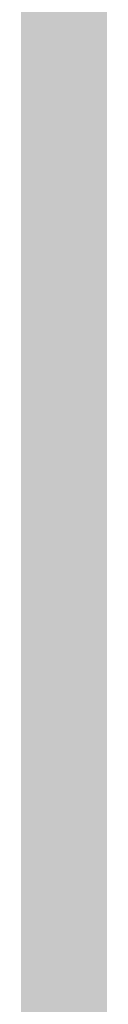
# Model space of a CAD drawing. Units: inches. Extents: x 2083 to 3317, y 1141 to 2115.
# Tile 189 of 256: x 3126.9283 to 3126.9467, y 1263.3548 to 1263.6134. Entities that reach past the tile are written whole.
import ezdxf

# ---------------------------------------------------------------- set-up
doc = ezdxf.new("R2010")
doc.units = ezdxf.units.IN
doc.layers.add('A-ANNO-DIMS', color=2, linetype='Continuous', lineweight=18)
doc.layers.add('A-WALL-PATT', color=251, linetype='Continuous', lineweight=13, true_color=0x636466)
doc.styles.get("Standard").update_dxf_attribs({"font": 'arial.ttf'})
doc.dimstyles.new('ISO-25', dxfattribs={"dimtxt": 12, "dimasz": 12, "dimexe": 1.25, "dimexo": 0.625, "dimtad": 1, "dimlunit": 3, "dimtxsty": 'Standard', "dimcen": 2.5, "dimadec": 0, "dimazin": 0, "dimtfac": 1, "dimtmove": 0, "dimatfit": 3, "dimfxl": 1, "dimarcsym": 0})

# ---------------------------------------------------------------- blocks, each defined once
blk = doc.blocks.new('*D26')
at = {"layer": 'A-ANNO-DIMS', "color": 0, "lineweight": -2, "transparency": 16777216}
for p, q in [((3088.98584, 1274.91509), (3088.98584, 1270.95196)), ((3111.24004, 1274.91509), (3111.24004, 1270.95196)), ((3076.98584, 1272.20196), (2840.26245, 1272.20196)), ((3111.24004, 1272.20196), (3088.98584, 1272.20196)), ((3123.24004, 1272.20196), (3135.24004, 1272.20196))]:
    blk.add_line(p, q, dxfattribs=at)
at = {"layer": 'A-ANNO-DIMS', "color": 0, "transparency": 16777216}
for points in [[(3076.98584, 1274.20196), (3076.98584, 1270.20196), (3088.98584, 1272.20196)], [(3123.24004, 1274.20196), (3123.24004, 1270.20196), (3111.24004, 1272.20196)]]:
    blk.add_solid(points, dxfattribs=at)
at = {"layer": 'Defpoints', "color": 0, "transparency": 16777216}
for p in [(3088.98584, 1275.54009), (3111.24004, 1275.54009), (3088.98584, 1272.20196)]:
    blk.add_point(p, dxfattribs=at)
at = {"layer": 'A-ANNO-DIMS', "color": 0, "transparency": 16777216, "insert": (2952.62415, 1279.0316), "char_height": 12, "attachment_point": 5}
blk.add_mtext('NIGHTSTAND 1\'-10 1/2" TYP.', dxfattribs=at)
blk = doc.blocks.new('*D27')
at = {"layer": 'A-ANNO-DIMS', "color": 0, "lineweight": -2, "transparency": 16777216}
for p, q in [((3114.57817, 1309.79428), (3114.57817, 1321.79428)), ((3111.86504, 1297.79428), (3115.82817, 1297.79428)), ((3114.57817, 1297.79428), (3114.57817, 1275.54009)), ((3111.86504, 1275.54009), (3115.82817, 1275.54009)), ((3114.57817, 1263.54009), (3114.57817, 1140.98859))]:
    blk.add_line(p, q, dxfattribs=at)
at = {"layer": 'A-ANNO-DIMS', "color": 0, "transparency": 16777216}
for points in [[(3112.57817, 1309.79428), (3116.57817, 1309.79428), (3114.57817, 1297.79428)], [(3112.57817, 1263.54009), (3116.57817, 1263.54009), (3114.57817, 1275.54009)]]:
    blk.add_solid(points, dxfattribs=at)
at = {"layer": 'Defpoints', "color": 0, "transparency": 16777216}
for p in [(3111.24004, 1297.79428), (3111.24004, 1275.54009), (3114.57817, 1275.54009)]:
    blk.add_point(p, dxfattribs=at)
at = {"layer": 'A-ANNO-DIMS', "color": 0, "transparency": 16777216, "insert": (3107.74853, 1196.26434), "char_height": 12, "attachment_point": 5, "rotation": 90}
blk.add_mtext('1\'-10 1/2" TYP.', dxfattribs=at)

msp = doc.modelspace()

# ---------------------------------------------------------------- hatches: boundary and pattern name
at = {"layer": 'A-WALL-PATT'}
h = msp.add_hatch(color=256, dxfattribs=at)
h.dxf.hatch_style = 1
h.paths.add_polyline_path([(3126.95978, 2020.76136), (2748.95978, 2020.76136), (2604.95978, 2020.76136), (2226.95978, 2020.76136), (2226.95978, 1702.76136), (2466.95978, 1702.76136), (2466.95978, 1582.76136), (2418.95978, 1582.76136), (2418.95978, 1477.76136), (2226.95978, 1477.76136), (2226.95978, 1263.26136), (2544.95978, 1263.26136), (2544.95978, 1411.76136), (2604.95978, 1411.76136), (2685.95978, 1411.76136), (2685.95978, 1420.76136), (2604.95978, 1420.76136), (2604.95978, 1573.76136), (2604.95978, 1702.76136), (2604.95978, 2011.76136), (2748.95978, 2011.76136), (2748.95978, 1702.76136), (2862.95978, 1702.76136), (2862.95978, 1621.76136), (2871.95978, 1621.76136), (2871.95978, 1702.76136), (2883.95978, 1702.76136), (2883.95978, 1706.93946, -0.026459), (2883.95978, 1711.76136), (2757.95978, 1711.76136), (2757.95978, 1807.76136), (2787.95978, 1807.76136), (2787.95978, 1812.26136), (2757.95978, 1812.26136), (2757.95978, 2011.76136), (2877.95978, 2011.76136), (2877.95978, 1812.26136), (2847.95978, 1812.26136), (2847.95978, 1807.76136), (2889.83574, 1807.76136), (2889.83574, 1812.26136), (2882.45978, 1812.26136), (2882.45978, 2011.76136), (3117.95978, 2011.76136), (3117.95978, 1812.26136), (2937.83574, 1812.26136), (2937.83574, 1807.76136), (2995.70978, 1807.76136), (2995.70978, 1796.11767), (3000.20978, 1796.11767), (3000.20978, 1807.76136), (3117.95978, 1807.76136), (3117.95978, 1711.76136), (3000.20978, 1711.76136), (3000.20978, 1760.11767), (2998.5727, 1760.11767, -0.020711), (2995.70978, 1760.11767), (2995.70978, 1711.76136), (2931.95978, 1711.76136), (2931.95978, 1702.76136), (3126.95978, 1702.76136)])
h.paths.add_polyline_path([(2471.45978, 2011.76136), (2471.45978, 1810.01136), (2462.71694, 1810.01136), (2462.71694, 1805.51136), (2505.95978, 1805.51136), (2505.95978, 1810.01136), (2475.95978, 1810.01136), (2475.95978, 2011.76136), (2595.95978, 2011.76136), (2595.95978, 1810.01136), (2565.95978, 1810.01136), (2565.95978, 1805.51136), (2595.95978, 1805.51136), (2595.95978, 1711.76136), (2235.95978, 1711.76136), (2235.95978, 1805.51136), (2353.70978, 1805.51136), (2353.70978, 1796.05416), (2358.20978, 1796.05416), (2358.20978, 1805.51136), (2414.71694, 1805.51136), (2414.71694, 1810.01136), (2235.95978, 1810.01136), (2235.95978, 2011.76136)], flags=16)
h.paths.add_polyline_path([(2270.20473, 1994.61001), (2270.20473, 1970.61001), (2246.20473, 1970.61001), (2246.20473, 1994.61001)], flags=0)
edge = h.paths.add_edge_path(flags=0)
edge.add_ellipse((2332.02739, 1899.79818), major_axis=(-3.04299, 3.04299), ratio=0.1682525, start_angle=-161.33217, end_angle=-156.30711, ccw=False)
edge.add_ellipse((2333.08204, 1898.74353), major_axis=(-1.05465, 1.05465), ratio=0.4535321, start_angle=-123.37102, end_angle=-94.15911)
edge = h.paths.add_edge_path(flags=0)
edge.add_ellipse((2332.02739, 1968.87629), major_axis=(3.04299, 3.04299), ratio=0.1682525, start_angle=18.66783, end_angle=23.69289)
edge.add_spline(control_points=[(2332.9256, 1970.6911), (2332.22677, 1970.3361), (2330.89371, 1969.65891), (2328.41308, 1970.93214), (2327.20393, 1967.74871), (2324.7096, 1969.95559), (2322.53282, 1967.01235), (2320.01285, 1971.29581), (2317.68031, 1968.15784), (2316.04053, 1967.10205), (2315.4269, 1966.8096)], knot_values=[0, 0, 0, 0, 2.267059, 4.324559, 6.685584, 8.878641, 11.121502, 14.300359, 17.755284, 19.732645, 19.732645, 19.732645, 19.732645], degree=3, periodic=0)
edge.add_ellipse((2332.02739, 1968.87629), major_axis=(3.04299, 3.04299), ratio=0.1682525, start_angle=18.66783, end_angle=23.69289, ccw=False)
edge.add_ellipse((2333.08204, 1969.93094), major_axis=(1.05465, 1.05465), ratio=0.4535321, start_angle=56.62898, end_angle=85.84089, ccw=False)
edge = h.paths.add_edge_path(flags=0)
edge.add_spline(control_points=[(2296.42829, 1967.98791), (2293.6278, 1965.33631), (2287.70362, 1959.72709), (2299.74386, 1949.9957), (2294.53259, 1935.66853), (2290.57323, 1920.60351), (2293.39412, 1909.97369), (2296.18541, 1904.96654)], knot_values=[0.099185, 0.099185, 0.099185, 0.099185, 0.345301, 0.619822, 0.982653, 1.386093, 1.810555, 1.810555, 1.810555, 1.810555], degree=3, periodic=0)
edge.add_spline(control_points=[(2296.18541, 1904.96654), (2297.38358, 1902.6193), (2298.00097, 1901.94931), (2298.55297, 1901.46815)], knot_values=[0.006246, 0.006246, 0.006246, 0.006246, 0.055476, 0.055476, 0.055476, 0.055476], degree=3, periodic=0)
edge.add_spline(control_points=[(2298.55297, 1901.46815), (2297.25861, 1900.92322), (2295.22529, 1900.23213), (2293.06023, 1900.61421), (2292.10142, 1900.78841), (2292.08958, 1900.79057)], knot_values=[0.312835, 0.312835, 0.312835, 0.312835, 0.40178, 0.474987, 0.475903, 0.475903, 0.475903, 0.475903], degree=3, periodic=0)
edge.add_arc((2292.79365, 1904.66411), 3.93701, 215.4209, 259.69818, ccw=False)
edge.add_spline(control_points=[(2289.58531, 1902.3823), (2289.47665, 1902.53509), (2289.36848, 1902.68804), (2289.26086, 1902.84117)], knot_values=[0.102872, 0.102872, 0.102872, 0.102872, 0.116896, 0.116896, 0.116896, 0.116896], degree=3, periodic=0)
edge.add_spline(control_points=[(2289.26086, 1902.84117), (2288.6866, 1902.55019), (2287.64005, 1902.0199), (2285.88134, 1901.87395), (2283.85297, 1901.50435), (2281.71999, 1899.71054), (2278.46699, 1899.49294), (2276.15714, 1901.8832), (2272.25895, 1899.80407), (2267.77761, 1901.84318), (2262.24388, 1900.18403), (2257.41493, 1901.78206), (2254.31837, 1900.72612), (2253.17828, 1900.33734)], knot_values=[0, 0, 0, 0, 1.907977, 3.477176, 5.261074, 7.972851, 11.680248, 13.717921, 16.939592, 22.789562, 27.502503, 33.595215, 37.145618, 37.145618, 37.145618, 37.145618], degree=3, periodic=0)
edge.add_line((2253.17828, 1900.33734), (2250.24424, 1902.84117))
edge.add_line((2250.24424, 1902.84117), (2250.24424, 1965.8333))
edge.add_line((2250.24424, 1965.8333), (2253.17828, 1968.33712))
edge.add_spline(control_points=[(2253.17828, 1968.33712), (2254.31837, 1967.94835), (2257.41493, 1966.89241), (2262.24388, 1968.49043), (2267.77761, 1966.83128), (2271.52673, 1968.53722), (2273.87591, 1967.82829), (2274.2067, 1967.72764)], knot_values=[0, 0, 0, 0, 0.09018, 0.244935, 0.364644, 0.513233, 0.537855, 0.537855, 0.537855, 0.537855], degree=3, periodic=0)
edge.add_arc((2274.35289, 1963.79335), 3.93701, 72.05113, 92.12795, ccw=False)
edge.add_arc((2281.29693, 1985.23), 18.5963, 252.051134, 288.565722)
edge.add_arc((2292.31672, 1956.02888), 12.64608, 71.026788, 113.778218, ccw=False)
edge = h.paths.add_edge_path(flags=0)
edge.add_spline(control_points=[(2274.89941, 1951.85619), (2275.06616, 1951.61659), (2275.23269, 1951.37659), (2275.39799, 1951.13585)], knot_values=[1.409916, 1.409916, 1.409916, 1.409916, 1.43159, 1.43159, 1.43159, 1.43159], degree=3, periodic=0)
edge.add_spline(control_points=[(2275.39799, 1951.13585), (2275.79211, 1950.56189), (2276.17923, 1949.98377), (2276.54555, 1949.3971)], knot_values=[1.358238, 1.358238, 1.358238, 1.358238, 1.409916, 1.409916, 1.409916, 1.409916], degree=3, periodic=0)
edge.add_line((2276.54555, 1949.3971), (2277.43729, 1947.86218))
edge.add_spline(control_points=[(2277.43729, 1947.86218), (2276.30383, 1945.67311), (2274.6397, 1942.42688), (2274.63161, 1938.0939), (2272.79912, 1930.85155), (2274.35643, 1943.89705), (2275.94768, 1947.92336), (2276.54555, 1949.3971)], knot_values=[0.005632, 0.005632, 0.005632, 0.005632, 0.186014, 0.266002, 0.357087, 0.59639, 0.739732, 0.739732, 0.739732, 0.739732], degree=3, periodic=0)
edge.add_spline(control_points=[(2276.54555, 1949.3971), (2276.17923, 1949.98377), (2275.79211, 1950.56189), (2275.39799, 1951.13585)], knot_values=[1.358238, 1.358238, 1.358238, 1.358238, 1.409916, 1.409916, 1.409916, 1.409916], degree=3, periodic=0)
edge.add_spline(control_points=[(2275.39799, 1951.13585), (2274.9425, 1950.08045), (2274.20776, 1948.02527), (2273.9346, 1944.85148), (2272.46853, 1937.62749), (2273.46622, 1945.69647), (2274.70062, 1951.05947), (2274.89941, 1951.85619)], knot_values=[0.104364, 0.104364, 0.104364, 0.104364, 0.189636, 0.269624, 0.36071, 0.600013, 0.644622, 0.644622, 0.644622, 0.644622], degree=3, periodic=0)
h.paths.add_polyline_path([(2269.16751, 1963.12757, -0.357527), (2268.17063, 1960.97637, -0.092561), (2268.17063, 1939.43632, -0.357527), (2269.16751, 1937.28512, -0.357527), (2267.01631, 1938.282, -0.164785), (2254.68558, 1938.282, -0.357527), (2252.53438, 1937.28512, -0.357527), (2253.53126, 1939.43632, -0.092561), (2253.53126, 1960.97637, -0.357527), (2252.53438, 1963.12757, -0.357527), (2254.68558, 1962.13069, -0.164785), (2267.01631, 1962.13069, -0.357527)], flags=0)
h.paths.add_polyline_path([(2248.87407, 1967.8018), (2248.87407, 1957.02771), (2249.45778, 1957.02771), (2249.45778, 1911.64676), (2248.87407, 1911.64676), (2248.87407, 1900.87267), (2246.51186, 1900.87267, 0.197327), (2244.14966, 1902.45687), (2244.14966, 1966.21759, 0.197327), (2246.51186, 1967.8018)], flags=0)
h.paths.add_polyline_path([(2269.16751, 1931.38934, -0.357527), (2268.17063, 1929.23814, -0.092561), (2268.17063, 1907.6981, -0.357527), (2269.16751, 1905.54689, -0.357527), (2267.01631, 1906.54377, -0.164785), (2254.68558, 1906.54377, -0.357527), (2252.53438, 1905.54689, -0.357527), (2253.53126, 1907.6981, -0.092561), (2253.53126, 1929.23814, -0.357527), (2252.53438, 1931.38934, -0.357527), (2254.68558, 1930.39246, -0.164785), (2267.01631, 1930.39246, -0.357527)], flags=0)
edge = h.paths.add_edge_path(flags=0)
edge.add_spline(control_points=[(2276.19686, 1906.7237), (2276.16814, 1909.02893), (2276.11405, 1913.37185), (2270.59842, 1924.92498), (2273.90517, 1919.01278), (2275.92171, 1916.26206), (2275.47457, 1912.40215), (2277.25787, 1910.38062), (2276.69604, 1908.22504), (2276.64622, 1906.81302), (2276.61782, 1906.00841)], knot_values=[0, 0, 0, 0, 8.61026, 16.221274, 18.843057, 23.804898, 27.440828, 29.356102, 31.203478, 33.650687, 33.650687, 33.650687, 33.650687], degree=3, periodic=0)
edge.add_spline(control_points=[(2276.61782, 1906.00841), (2276.62331, 1905.62414), (2276.49774, 1904.62866), (2275.44178, 1903.85473), (2274.93731, 1903.08045), (2274.85908, 1902.84117)], knot_values=[0.156488, 0.156488, 0.156488, 0.156488, 0.184398, 0.231376, 0.250598, 0.250598, 0.250598, 0.250598], degree=3, periodic=0)
edge.add_line((2274.85908, 1902.84117), (2276.50598, 1902.84117))
edge.add_spline(control_points=[(2276.50598, 1902.84117), (2276.78831, 1903.08494), (2277.66507, 1904.1252), (2278.24954, 1904.34074), (2277.65387, 1908.52739), (2278.15567, 1906.22781), (2278.10046, 1905.28595), (2278.84667, 1904.06901), (2277.85679, 1903.41495), (2277.87419, 1902.99105), (2277.90356, 1902.84117)], knot_values=[0.059574, 0.059574, 0.059574, 0.059574, 0.080753, 0.103741, 0.16972, 0.176036, 0.207137, 0.240474, 0.262341, 0.27366, 0.27366, 0.27366, 0.27366], degree=3, periodic=0)
edge.add_line((2277.90356, 1902.84117), (2280.02983, 1902.84117))
edge.add_spline(control_points=[(2280.02983, 1902.84117), (2279.88822, 1903.0884), (2279.49926, 1903.98155), (2280.15228, 1905.93935), (2278.10362, 1909.65776), (2279.76239, 1907.18529), (2280.3279, 1904.87486), (2280.48511, 1903.48959), (2281.46327, 1903.24943), (2281.75834, 1902.9365), (2281.83404, 1902.84117)], knot_values=[0.013856, 0.013856, 0.013856, 0.013856, 0.034874, 0.088867, 0.107879, 0.126738, 0.158714, 0.193757, 0.217487, 0.226722, 0.226722, 0.226722, 0.226722], degree=3, periodic=0)
edge.add_spline(control_points=[(2281.83404, 1902.84117), (2281.78753, 1902.8267), (2281.64702, 1902.78299), (2281.39553, 1902.85949), (2281.08808, 1902.98524), (2280.72068, 1903.0609), (2280.33345, 1903.02573), (2280.12477, 1902.89888), (2280.02983, 1902.84117)], knot_values=[0, 0, 0, 0, 0.14413, 0.435517, 0.749276, 1.153046, 1.548371, 1.878348, 1.878348, 1.878348, 1.878348], degree=3, periodic=0)
edge.add_line((2280.02983, 1902.84117), (2277.90356, 1902.84117))
edge.add_spline(control_points=[(2277.90356, 1902.84117), (2277.89286, 1902.79586), (2277.8654, 1902.67964), (2277.60748, 1902.68748), (2277.27405, 1902.8007), (2276.83792, 1902.61977), (2276.58381, 1902.78926), (2276.50598, 1902.84117)], knot_values=[0, 0, 0, 0, 0.127189, 0.326199, 0.628009, 1.24357, 1.515331, 1.515331, 1.515331, 1.515331], degree=3, periodic=0)
edge.add_line((2276.50598, 1902.84117), (2274.85908, 1902.84117))
edge.add_spline(control_points=[(2274.85908, 1902.84117), (2274.81444, 1902.89859), (2274.72513, 1903.01345), (2274.49348, 1903.11897), (2274.24429, 1902.96054), (2273.93712, 1903.18494), (2273.61404, 1902.98314), (2273.40832, 1902.88304), (2273.32225, 1902.84117)], knot_values=[0, 0, 0, 0, 0.21843, 0.436957, 0.687977, 0.990379, 1.398396, 1.69185, 1.69185, 1.69185, 1.69185], degree=3, periodic=0)
edge.add_spline(control_points=[(2273.32225, 1902.84117), (2273.61674, 1903.44569), (2274.274, 1904.53825), (2276.02724, 1904.5737), (2276.20696, 1906.58364), (2276.19686, 1906.7237)], knot_values=[0.012227, 0.012227, 0.012227, 0.012227, 0.059472, 0.106218, 0.134458, 0.134458, 0.134458, 0.134458], degree=3, periodic=0)
h.paths.add_polyline_path([(2270.77605, 1897.78983), (2270.77605, 1873.78983), (2246.77605, 1873.78983), (2246.77605, 1897.78983)], flags=0)
h.paths.add_polyline_path([(2353.70978, 1760.00506), (2353.70978, 1760.05416), (2358.20978, 1760.05416, -0.033729)], flags=0)
h.paths.add_polyline_path([(2321.81912, 1737.52919), (2341.99533, 1737.52919, -0.414214), (2343.20327, 1736.32124), (2343.20327, 1721.0206, -0.414214), (2341.99533, 1719.81265), (2321.81912, 1719.81265, -0.414214), (2320.61117, 1721.0206), (2320.61117, 1736.32124, -0.414214)], flags=0)
h.paths.add_polyline_path([(2324.23501, 1736.32124), (2339.57944, 1736.32124, -0.414214), (2341.99533, 1733.90535), (2341.99533, 1725.44973, -0.414214), (2339.57944, 1723.03384), (2333.68059, 1723.03384), (2333.84532, 1722.04547, -0.870646), (2335.4254, 1721.82589, -0.767327), (2333.92269, 1721.42324), (2331.29102, 1721.42324, -0.767327), (2329.78832, 1721.82589, -0.870646), (2331.3684, 1722.04547), (2331.53313, 1723.03384), (2324.23501, 1723.03384, -0.414214), (2321.81912, 1725.44973), (2321.81912, 1733.90535, -0.414214)], flags=0)
h.paths.add_polyline_path([(2570.48379, 1928.61544), (2589.68379, 1928.61544), (2590.16883, 1928.61544), (2590.16883, 1904.9934), (2570.48379, 1904.9934)], flags=0)
h.paths.add_polyline_path([(2574.44732, 1927.26382, -1), (2572.82884, 1927.26382, -1)], flags=0)
h.paths.add_polyline_path([(2573.08987, 1926.94088), (2573.92503, 1927.77604), (2574.14774, 1927.55333), (2573.31258, 1926.71817)], flags=0)
h.paths.add_polyline_path([(2578.77906, 1919.72962, -1), (2571.59166, 1919.72962, -1)], flags=0)
h.paths.add_polyline_path([(2578.38536, 1919.72962, -1), (2571.98536, 1919.72962, -1)], flags=0)
h.paths.add_polyline_path([(2331.59576, 1729.47622, -1), (2333.61795, 1729.47622, -1)], flags=0)
h.paths.add_polyline_path([(2578.03423, 1927.26382, -1), (2576.41574, 1927.26382, -1)], flags=0)
h.paths.add_polyline_path([(2576.68885, 1927.53109), (2576.91156, 1927.7538), (2577.74673, 1926.91863), (2577.52402, 1926.69592)], flags=0)
h.paths.add_polyline_path([(2578.13906, 1909.85954, -1), (2572.23166, 1909.85954, -1)], flags=0)
h.paths.add_polyline_path([(2577.74536, 1909.85954, -1), (2572.62536, 1909.85954, -1)], flags=0)
h.paths.add_polyline_path([(2583.79772, 1927.26382, -1), (2582.17923, 1927.26382, -1)], flags=0)
h.paths.add_polyline_path([(2582.71865, 1927.7538), (2583.55381, 1926.91863), (2583.3311, 1926.69592), (2582.49594, 1927.53109)], flags=0)
h.paths.add_polyline_path([(2582.49594, 1927.53109), (2582.71865, 1927.7538), (2583.55381, 1926.91863), (2583.3311, 1926.69592)], flags=0)
h.paths.add_polyline_path([(2587.73906, 1920.52962, -1), (2581.83166, 1920.52962, -1)], flags=0)
h.paths.add_polyline_path([(2587.34536, 1920.52962, -1), (2582.22536, 1920.52962, -1)], flags=0)
h.paths.add_polyline_path([(2587.38462, 1927.26382, -1), (2585.76613, 1927.26382, -1)], flags=0)
h.paths.add_polyline_path([(2586.08199, 1926.98025), (2586.91716, 1927.81541), (2587.13987, 1927.5927), (2586.3047, 1926.75754)], flags=0)
h.paths.add_polyline_path([(2588.37906, 1910.65954, -1), (2581.19166, 1910.65954, -1)], flags=0)
h.paths.add_polyline_path([(2587.98536, 1910.65954, -1), (2581.58536, 1910.65954, -1)], flags=0)
h.paths.add_polyline_path([(2417.16773, 1729.4779), (2437.34394, 1729.4779, -0.414214), (2438.55188, 1728.26995), (2438.55188, 1712.96931, -0.414214), (2437.34394, 1711.76136), (2417.16773, 1711.76136, -0.414214), (2415.95978, 1712.96931), (2415.95978, 1728.26995, -0.414214)], flags=0)
h.paths.add_polyline_path([(2419.58362, 1728.26995), (2434.92805, 1728.26995, -0.414214), (2437.34394, 1725.85406), (2437.34394, 1717.39844, -0.414214), (2434.92805, 1714.98255), (2429.0292, 1714.98255), (2429.19393, 1713.99418, -0.870646), (2430.77401, 1713.7746, -0.767327), (2429.2713, 1713.37195), (2426.63963, 1713.37195, -0.767327), (2425.13693, 1713.7746, -0.870646), (2426.71701, 1713.99418), (2426.88174, 1714.98255), (2419.58362, 1714.98255, -0.414214), (2417.16773, 1717.39844), (2417.16773, 1725.85406, -0.414214)], flags=0)
h.paths.add_polyline_path([(2419.58362, 1728.26995), (2434.92805, 1728.26995, -0.414214), (2437.34394, 1725.85406), (2437.34394, 1717.39844, -0.414214), (2434.92805, 1714.98255), (2429.0292, 1714.98255), (2428.35812, 1719.00903), (2427.55282, 1719.00903), (2426.88174, 1714.98255), (2419.58362, 1714.98255, -0.414214), (2417.16773, 1717.39844), (2417.16773, 1725.85406, -0.414214)], flags=0)
h.paths.add_polyline_path([(2426.94437, 1721.42492, -1), (2428.96656, 1721.42492, -1)], flags=0)
h.paths.add_polyline_path([(2475.95978, 1702.76136), (2595.95978, 1702.76136), (2595.95978, 1582.76136), (2475.95978, 1582.76136)], flags=16)
h.paths.add_polyline_path([(2427.95978, 1573.76136), (2595.95978, 1573.76136), (2595.95978, 1468.76136), (2595.95978, 1420.76136), (2384.45978, 1420.76136), (2384.45978, 1468.76136), (2427.95978, 1468.76136)], flags=16)
h.paths.add_polyline_path([(2379.95978, 1468.76136), (2379.95978, 1420.76136), (2235.95978, 1420.76136), (2235.95978, 1468.76136)], flags=16)
h.paths.add_polyline_path([(2317.816, 1466.69577), (2337.9922, 1466.69577, -0.414214), (2339.20015, 1465.48782), (2339.20015, 1450.18718, -0.414214), (2337.9922, 1448.97923), (2317.816, 1448.97923, -0.414214), (2316.60805, 1450.18718), (2316.60805, 1465.48782, -0.414214)], flags=0)
h.paths.add_polyline_path([(2320.23189, 1465.48782), (2335.57631, 1465.48782, -0.414214), (2337.9922, 1463.07193), (2337.9922, 1454.61631, -0.414214), (2335.57631, 1452.20042), (2329.67747, 1452.20042), (2329.84219, 1451.21205, -0.870646), (2331.42228, 1450.99247, -0.767327), (2329.91957, 1450.58983), (2327.2879, 1450.58983, -0.767327), (2325.7852, 1450.99247, -0.870646), (2327.36528, 1451.21205), (2327.53001, 1452.20042), (2320.23189, 1452.20042, -0.414214), (2317.816, 1454.61631), (2317.816, 1463.07193, -0.414214)], flags=0)
h.paths.add_polyline_path([(2320.23189, 1465.48782), (2335.57631, 1465.48782, -0.414214), (2337.9922, 1463.07193), (2337.9922, 1454.61631, -0.414214), (2335.57631, 1452.20042), (2329.67747, 1452.20042), (2329.00638, 1456.22691), (2328.20109, 1456.22691), (2327.53001, 1452.20042), (2320.23189, 1452.20042, -0.414214), (2317.816, 1454.61631), (2317.816, 1463.07193, -0.414214)], flags=0)
h.paths.add_polyline_path([(2327.59264, 1458.6428, -1), (2329.61483, 1458.6428, -1)], flags=0)
h.paths.add_polyline_path([(2244.41174, 1433.34045), (2241.92094, 1433.34045, -0.414214), (2240.01786, 1435.24354), (2240.01786, 1440.95281, -0.414211), (2241.92093, 1442.8559), (2244.41174, 1442.8559, -1.976472)], flags=0)
h.paths.add_polyline_path([(2245.35689, 1434.39754, -0.414214), (2245.35689, 1441.79881, -2.144098)], flags=0)
h.paths.add_polyline_path([(2535.95978, 1416.26136), (2535.95978, 1272.26136), (2235.95978, 1272.26136), (2235.95978, 1416.26136)], flags=16)
h.paths.add_polyline_path([(2260.11956, 1384.29284), (2260.11956, 1362.03865), (2237.86537, 1362.03865), (2237.86537, 1384.29284)], flags=0)
edge = h.paths.add_edge_path(flags=0)
edge.add_line((2318.25185, 1362.0933), (2318.1458, 1362.00097))
edge.add_ellipse((2317.44512, 1360.43104), major_axis=(2.82164, 2.82164), ratio=0.1682525, start_angle=18.66783, end_angle=20.94813, ccw=False)
edge.add_ellipse((2318.42305, 1361.40897), major_axis=(0.97793, 0.97793), ratio=0.4535321, start_angle=56.62898, end_angle=70.2262, ccw=False)
edge = h.paths.add_edge_path(flags=0)
edge.add_line((2319.10737, 1295.57108), (2319.01504, 1295.67713))
edge.add_ellipse((2317.44512, 1296.37781), major_axis=(-2.82164, 2.82164), ratio=0.1682525, start_angle=-161.33217, end_angle=-159.05187, ccw=False)
edge.add_ellipse((2318.42305, 1295.39988), major_axis=(-0.97793, 0.97793), ratio=0.4535321, start_angle=-123.37102, end_angle=-109.7738)
edge = h.paths.add_edge_path(flags=0)
edge.add_spline(control_points=[(2284.21035, 1301.17022), (2284.58069, 1300.44472), (2284.89119, 1299.89202), (2285.15955, 1299.46102)], knot_values=[0.039066, 0.039066, 0.039066, 0.039066, 0.055476, 0.055476, 0.055476, 0.055476], degree=3, periodic=0)
edge.add_line((2285.15955, 1299.46102), (2284.21035, 1301.17022))
edge = h.paths.add_edge_path(flags=0)
edge.add_line((2280.41246, 1297.29801), (2283.36999, 1297.03612))
edge.add_line((2283.36999, 1297.03612), (2286.40569, 1297.92631))
edge.add_spline(control_points=[(2286.40569, 1297.92631), (2285.30549, 1297.46312), (2284.34478, 1297.12915), (2283.36999, 1297.03612)], knot_values=[0.394369, 0.394369, 0.394369, 0.394369, 0.475903, 0.475903, 0.475903, 0.475903], degree=3, periodic=0)
edge.add_spline(control_points=[(2283.36999, 1297.03612), (2283.28139, 1297.02767), (2282.31629, 1296.95734), (2281.3125, 1297.13448), (2280.42344, 1297.29602), (2280.41246, 1297.29801)], knot_values=[0.312835, 0.312835, 0.312835, 0.312835, 0.320246, 0.393453, 0.394369, 0.394369, 0.394369, 0.394369], degree=3, periodic=0)
edge = h.paths.add_edge_path(flags=0)
edge.add_line((2284.43556, 1359.60729), (2280.44629, 1355.32805))
edge.add_line((2280.44629, 1355.32805), (2279.57999, 1351.01775))
edge.add_line((2279.57999, 1351.01775), (2282.41297, 1346.58043))
edge.add_spline(control_points=[(2282.41297, 1346.58043), (2283.15333, 1345.58924), (2284.2529, 1344.0289), (2284.80104, 1342.38717), (2284.93516, 1341.80554)], knot_values=[1.240098, 1.240098, 1.240098, 1.240098, 1.332892, 1.382712, 1.382712, 1.382712, 1.382712], degree=3, periodic=0)
edge.add_spline(control_points=[(2284.93516, 1341.80554), (2285.31911, 1340.1406), (2285.23303, 1338.4092), (2284.90994, 1336.65412)], knot_values=[1.097484, 1.097484, 1.097484, 1.097484, 1.240098, 1.240098, 1.240098, 1.240098], degree=3, periodic=0)
edge.add_spline(control_points=[(2284.90994, 1336.65412), (2284.58685, 1334.89904), (2284.02675, 1333.12027), (2283.46264, 1331.36058)], knot_values=[0.95487, 0.95487, 0.95487, 0.95487, 1.097484, 1.097484, 1.097484, 1.097484], degree=3, periodic=0)
edge.add_line((2283.46264, 1331.36058), (2281.89038, 1326.15336))
edge.add_line((2281.89038, 1326.15336), (2280.75626, 1321.05609))
edge.add_line((2280.75626, 1321.05609), (2280.2992, 1316.00198))
edge.add_line((2280.2992, 1316.00198), (2280.71593, 1310.95007))
edge.add_line((2280.71593, 1310.95007), (2282.02809, 1305.97214))
edge.add_line((2282.02809, 1305.97214), (2284.21035, 1301.17022))
edge.add_spline(control_points=[(2284.21035, 1301.17022), (2283.34073, 1302.73019), (2282.6119, 1304.33649), (2282.02809, 1305.97214)], knot_values=[0.099185, 0.099185, 0.099185, 0.099185, 0.241799, 0.241799, 0.241799, 0.241799], degree=3, periodic=0)
edge.add_spline(control_points=[(2282.02809, 1305.97214), (2281.44428, 1307.60778), (2281.00549, 1309.27276), (2280.71593, 1310.95007)], knot_values=[0.241799, 0.241799, 0.241799, 0.241799, 0.384413, 0.384413, 0.384413, 0.384413], degree=3, periodic=0)
edge.add_spline(control_points=[(2280.71593, 1310.95007), (2280.43324, 1312.58761), (2280.28939, 1314.27696), (2280.29889, 1315.96203), (2280.2992, 1316.00198)], knot_values=[0.384413, 0.384413, 0.384413, 0.384413, 0.523647, 0.527028, 0.527028, 0.527028, 0.527028], degree=3, periodic=0)
edge.add_spline(control_points=[(2280.2992, 1316.00198), (2280.31233, 1317.68696), (2280.47787, 1319.36793), (2280.75626, 1321.05609)], knot_values=[0.527028, 0.527028, 0.527028, 0.527028, 0.669642, 0.669642, 0.669642, 0.669642], degree=3, periodic=0)
edge.add_spline(control_points=[(2280.75626, 1321.05609), (2281.03465, 1322.74425), (2281.42588, 1324.43961), (2281.89038, 1326.15336)], knot_values=[0.669642, 0.669642, 0.669642, 0.669642, 0.812256, 0.812256, 0.812256, 0.812256], degree=3, periodic=0)
edge.add_spline(control_points=[(2281.89038, 1326.15336), (2282.26438, 1327.53325), (2282.78787, 1329.26181), (2283.35275, 1331.01778), (2283.46264, 1331.36058)], knot_values=[0.812256, 0.812256, 0.812256, 0.812256, 0.927087, 0.95487, 0.95487, 0.95487, 0.95487], degree=3, periodic=0)
edge.add_line((2283.46264, 1331.36058), (2284.90994, 1336.65412))
edge.add_line((2284.90994, 1336.65412), (2284.93516, 1341.80554))
edge.add_line((2284.93516, 1341.80554), (2282.41297, 1346.58043))
edge.add_spline(control_points=[(2282.41297, 1346.58043), (2281.27513, 1348.10379), (2280.07845, 1349.57032), (2279.57999, 1351.01775)], knot_values=[1.382712, 1.382712, 1.382712, 1.382712, 1.525326, 1.525326, 1.525326, 1.525326], degree=3, periodic=0)
edge.add_spline(control_points=[(2279.57999, 1351.01775), (2279.44328, 1351.41472), (2279.13631, 1352.85692), (2279.73519, 1354.29039), (2280.44629, 1355.32805)], knot_values=[1.525326, 1.525326, 1.525326, 1.525326, 1.564439, 1.667941, 1.667941, 1.667941, 1.667941], degree=3, periodic=0)
edge.add_spline(control_points=[(2280.44629, 1355.32805), (2281.42611, 1356.75784), (2282.93084, 1358.18256), (2284.43556, 1359.60729)], knot_values=[1.667941, 1.667941, 1.667941, 1.667941, 1.810555, 1.810555, 1.810555, 1.810555], degree=3, periodic=0)
edge.add_arc((2280.62307, 1348.51818), 11.72618, 71.026788, 113.778218)
edge.add_arc((2270.40489, 1375.59516), 17.24357, 252.051134, 288.565722, ccw=False)
edge.add_arc((2263.96597, 1355.71785), 3.65062, 72.05113, 92.12795)
edge.add_arc((2263.96597, 1355.71785), 3.65062, 92.12795, 177.98513)
edge.add_spline(control_points=[(2260.3176, 1355.8462), (2260.26042, 1354.22067), (2260.55128, 1350.18655), (2262.99934, 1346.76625), (2264.47274, 1344.64902)], knot_values=[1.43159, 1.43159, 1.43159, 1.43159, 1.564144, 1.770695, 1.770695, 1.770695, 1.770695], degree=3, periodic=0)
edge.add_line((2264.47274, 1344.64902), (2264.93559, 1343.98253))
edge.add_spline(control_points=[(2263.80104, 1340.24811), (2263.84324, 1340.51409), (2264.06724, 1341.75647), (2264.51269, 1343.00245), (2264.93505, 1343.98108)], knot_values=[0.53657, 0.53657, 0.53657, 0.53657, 0.559349, 0.644622, 0.644622, 0.644622, 0.644622], degree=3, periodic=0)
edge.add_spline(control_points=[(2264.93505, 1343.98108), (2265.11777, 1343.71497), (2265.29888, 1343.44791), (2265.47676, 1343.17936)], knot_values=[1.384077, 1.384077, 1.384077, 1.384077, 1.409916, 1.409916, 1.409916, 1.409916], degree=3, periodic=0)
edge.add_spline(control_points=[(2265.47676, 1343.17936), (2265.65464, 1342.91082), (2265.8293, 1342.64081), (2265.99913, 1342.36881)], knot_values=[1.358238, 1.358238, 1.358238, 1.358238, 1.384077, 1.384077, 1.384077, 1.384077], degree=3, periodic=0)
edge.add_line((2265.99913, 1342.36881), (2266.82601, 1340.94555))
edge.add_spline(control_points=[(2266.82601, 1340.94555), (2268.8944, 1337.08969), (2271.39817, 1325.843), (2270.51616, 1310.56856), (2275.91938, 1301.86061), (2277.78951, 1299.19945)], knot_values=[0.116896, 0.116896, 0.116896, 0.116896, 0.472987, 1.050969, 1.313793, 1.313793, 1.313793, 1.313793], degree=3, periodic=0)
edge.add_spline(control_points=[(2277.78951, 1299.19945), (2277.83941, 1299.12845), (2277.88943, 1299.0575), (2277.93957, 1298.98658)], knot_values=[0.109884, 0.109884, 0.109884, 0.109884, 0.116896, 0.116896, 0.116896, 0.116896], degree=3, periodic=0)
edge.add_line((2277.93957, 1298.98658), (2277.78885, 1299.19911))
edge.add_spline(control_points=[(2277.78885, 1299.19911), (2277.25658, 1298.92941), (2276.28635, 1298.4379), (2275.03935, 1298.33442), (2274.38333, 1298.2389), (2274.21525, 1298.20934)], knot_values=[33.12187, 33.12187, 33.12187, 33.12187, 35.029056, 36.598255, 37.144827, 37.144827, 37.144827, 37.144827], degree=3, periodic=0)
edge.add_line((2274.21525, 1298.20934), (2273.07315, 1297.89296))
edge.add_spline(control_points=[(2273.07315, 1297.89296), (2272.32294, 1297.57978), (2271.03915, 1296.51051), (2269.24839, 1296.22606), (2268.4231, 1296.37465)], knot_values=[26.532584, 26.532584, 26.532584, 26.532584, 29.198919, 31.839101, 31.839101, 31.839101, 31.839101], degree=3, periodic=0)
edge.add_line((2268.4231, 1296.37465), (2263.8785, 1297.45753))
edge.add_spline(control_points=[(2263.8785, 1297.45753), (2263.55608, 1297.35943), (2261.86031, 1296.83869), (2260.23878, 1297.28241), (2258.93345, 1297.51646)], knot_values=[15.919551, 15.919551, 15.919551, 15.919551, 16.939592, 21.226067, 21.226067, 21.226067, 21.226067], degree=3, periodic=0)
edge.add_line((2258.93345, 1297.51646), (2254.05523, 1297.32901))
edge.add_spline(control_points=[(2254.05523, 1297.32901), (2253.75553, 1297.29582), (2252.11368, 1297.16517), (2250.46187, 1297.54422), (2249.12969, 1297.66788)], knot_values=[5.306517, 5.306517, 5.306517, 5.306517, 6.276435, 10.613034, 10.613034, 10.613034, 10.613034], degree=3, periodic=0)
edge.add_line((2249.12969, 1297.66788), (2244.33165, 1296.87776))
edge.add_line((2244.33165, 1296.87776), (2241.61103, 1299.19945))
edge.add_line((2241.61103, 1299.19945), (2241.61103, 1357.6094))
edge.add_line((2241.61103, 1357.6094), (2244.33165, 1359.9311))
edge.add_line((2244.33165, 1359.9311), (2252.72882, 1359.54269))
edge.add_spline(control_points=[(2252.72882, 1359.54269), (2252.87094, 1359.54644), (2253.30574, 1359.54817), (2253.73984, 1359.51427), (2254.03174, 1359.48243)], knot_values=[0.233291, 0.233291, 0.233291, 0.233291, 0.244935, 0.268927, 0.268927, 0.268927, 0.268927], degree=3, periodic=0)
edge.add_line((2254.03174, 1359.48243), (2259.58719, 1359.41639))
edge.add_spline(control_points=[(2259.58719, 1359.41639), (2260.67707, 1359.6285), (2262.0732, 1359.897), (2263.52369, 1359.45928), (2263.83042, 1359.36595)], knot_values=[0.422516, 0.422516, 0.422516, 0.422516, 0.513233, 0.537855, 0.537855, 0.537855, 0.537855], degree=3, periodic=0)
edge.add_arc((2263.96597, 1355.71785), 3.65062, 72.05113, 92.12795, ccw=False)
edge.add_arc((2270.40489, 1375.59516), 17.24357, 252.051134, 288.565722)
edge.add_arc((2280.62307, 1348.51818), 11.72618, 71.026788, 113.778218, ccw=False)
h.paths.add_polyline_path([(2240.34053, 1359.43471), (2240.34053, 1349.44435), (2240.88178, 1349.44435), (2240.88178, 1307.3645), (2240.34053, 1307.3645), (2240.34053, 1297.37414), (2238.15016, 1297.37414, 0.197327), (2235.95978, 1298.84311), (2235.95978, 1357.96575, 0.197327), (2238.15016, 1359.43471)], flags=0)
h.paths.add_polyline_path([(2259.15779, 1355.1005, -0.357527), (2258.23342, 1353.10578, -0.092561), (2258.23342, 1333.1326, -0.357527), (2259.15779, 1331.13788, -0.357527), (2257.16307, 1332.06225, -0.164785), (2245.7293, 1332.06225, -0.357527), (2243.73458, 1331.13788, -0.357527), (2244.65895, 1333.1326, -0.092561), (2244.65895, 1353.10578, -0.357527), (2243.73458, 1355.1005, -0.357527), (2245.7293, 1354.17613, -0.164785), (2257.16307, 1354.17613, -0.357527)], flags=0)
edge = h.paths.add_edge_path(flags=0)
edge.add_line((2265.99913, 1342.36881), (2266.82601, 1340.94555))
edge.add_line((2266.82601, 1340.94555), (2265.30756, 1337.81407))
edge.add_line((2265.30756, 1337.81407), (2264.35823, 1334.65294))
edge.add_line((2264.35823, 1334.65294), (2264.26201, 1333.7997))
edge.add_spline(control_points=[(2264.26201, 1333.7997), (2264.20836, 1333.18705), (2264.16206, 1332.36553), (2264.00714, 1331.41393), (2263.96905, 1331.20183)], knot_values=[0.464444, 0.464444, 0.464444, 0.464444, 0.516691, 0.531608, 0.531608, 0.531608, 0.531608], degree=3, periodic=0)
edge.add_spline(control_points=[(2263.96905, 1331.20183), (2263.77453, 1330.11887), (2263.42437, 1328.79084), (2263.25742, 1328.53065), (2263.23403, 1328.51461)], knot_values=[0.372682, 0.372682, 0.372682, 0.372682, 0.44885, 0.464444, 0.464444, 0.464444, 0.464444], degree=3, periodic=0)
edge.add_spline(control_points=[(2263.23403, 1328.51461), (2263.09638, 1328.42023), (2263.13117, 1329.30148), (2263.27495, 1330.61575)], knot_values=[0.280919, 0.280919, 0.280919, 0.280919, 0.372682, 0.372682, 0.372682, 0.372682], degree=3, periodic=0)
edge.add_spline(control_points=[(2263.27495, 1330.61575), (2263.41874, 1331.93002), (2263.67152, 1333.67732), (2263.96985, 1335.31503)], knot_values=[0.189157, 0.189157, 0.189157, 0.189157, 0.280919, 0.280919, 0.280919, 0.280919], degree=3, periodic=0)
edge.add_spline(control_points=[(2263.96985, 1335.31503), (2264.1005, 1336.03219), (2264.41878, 1337.62191), (2264.75485, 1338.86443), (2264.94742, 1339.49112)], knot_values=[0.097394, 0.097394, 0.097394, 0.097394, 0.137578, 0.189157, 0.189157, 0.189157, 0.189157], degree=3, periodic=0)
edge.add_spline(control_points=[(2264.94742, 1339.49112), (2265.29002, 1340.60605), (2265.64424, 1341.494), (2265.99913, 1342.36881)], knot_values=[0.005632, 0.005632, 0.005632, 0.005632, 0.097394, 0.097394, 0.097394, 0.097394], degree=3, periodic=0)
h.paths.add_polyline_path([(2259.15779, 1325.67097, -0.357527), (2258.23342, 1323.67625, -0.092561), (2258.23342, 1303.70307, -0.357527), (2259.15779, 1301.70835, -0.357527), (2257.16307, 1302.63272, -0.164785), (2245.7293, 1302.63272, -0.357527), (2243.73458, 1301.70835, -0.357527), (2244.65895, 1303.70307, -0.092561), (2244.65895, 1323.67625, -0.357527), (2243.73458, 1325.67097, -0.357527), (2245.7293, 1324.74661, -0.164785), (2257.16307, 1324.74661, -0.357527)], flags=0)
edge = h.paths.add_edge_path(flags=0)
edge.add_spline(control_points=[(2261.70894, 1317.31142), (2261.67948, 1317.41758), (2261.76186, 1317.38853), (2262.49074, 1316.08987), (2262.96218, 1315.3009)], knot_values=[14.955861, 14.955861, 14.955861, 14.955861, 16.221274, 18.694826, 18.694826, 18.694826, 18.694826], degree=3, periodic=0)
edge.add_spline(control_points=[(2262.96218, 1315.3009), (2262.99044, 1315.25362), (2263.7021, 1314.06738), (2264.34898, 1313.12715), (2264.73005, 1312.16415)], knot_values=[18.694826, 18.694826, 18.694826, 18.694826, 18.843057, 22.433791, 22.433791, 22.433791, 22.433791], degree=3, periodic=0)
edge.add_spline(control_points=[(2264.73005, 1312.16415), (2264.87556, 1311.79644), (2265.17687, 1310.76981), (2265.14307, 1309.55926), (2265.24774, 1308.82419)], knot_values=[22.433791, 22.433791, 22.433791, 22.433791, 23.804898, 26.172756, 26.172756, 26.172756, 26.172756], degree=3, periodic=0)
edge.add_line((2265.24774, 1308.82419), (2265.85077, 1307.17189))
edge.add_spline(control_points=[(2265.85077, 1307.17189), (2266.06502, 1306.82168), (2266.38439, 1306.33225), (2266.4244, 1305.78055), (2266.42037, 1305.61122)], knot_values=[28.062562, 28.062562, 28.062562, 28.062562, 29.356102, 29.911721, 29.911721, 29.911721, 29.911721], degree=3, periodic=0)
edge.add_spline(control_points=[(2266.42037, 1305.61122), (2266.41612, 1305.43259), (2266.394, 1305.25), (2266.36478, 1305.06586)], knot_values=[29.911721, 29.911721, 29.911721, 29.911721, 30.497837, 30.497837, 30.497837, 30.497837], degree=3, periodic=0)
edge.add_line((2266.36478, 1305.06586), (2266.06615, 1302.1363))
edge.add_spline(control_points=[(2266.06615, 1302.1363), (2266.07124, 1301.77998), (2265.99808, 1301.19998), (2265.66327, 1300.75896), (2265.50891, 1300.58588)], knot_values=[0.156488, 0.156488, 0.156488, 0.156488, 0.184398, 0.203543, 0.203543, 0.203543, 0.203543], degree=3, periodic=0)
edge.add_line((2265.50891, 1300.58588), (2264.43534, 1299.19945))
edge.add_line((2264.43534, 1299.19945), (2265.96244, 1299.19945))
edge.add_line((2265.96244, 1299.19945), (2267.33599, 1301.17528))
edge.add_line((2267.33599, 1301.17528), (2267.31167, 1301.98624))
edge.add_spline(control_points=[(2267.31167, 1301.98624), (2267.26111, 1302.8624), (2267.16021, 1303.73713), (2267.27149, 1303.3259)], knot_values=[0.126229, 0.126229, 0.126229, 0.126229, 0.166617, 0.166617, 0.166617, 0.166617], degree=3, periodic=0)
edge.add_spline(control_points=[(2267.27149, 1303.3259), (2267.28003, 1303.2943), (2267.30979, 1303.17537), (2267.37345, 1302.88361), (2267.40612, 1302.68283), (2267.41793, 1302.60103)], knot_values=[0.166617, 0.166617, 0.166617, 0.166617, 0.16972, 0.176036, 0.180765, 0.180765, 0.180765, 0.180765], degree=3, periodic=0)
edge.add_spline(control_points=[(2267.74389, 1300.9875), (2267.68758, 1301.15094), (2267.48052, 1301.65666), (2267.48375, 1302.14479), (2267.41793, 1302.60103)], knot_values=[0.180765, 0.180765, 0.180765, 0.180765, 0.193767, 0.220139, 0.220139, 0.220139, 0.220139], degree=3, periodic=0)
edge.add_line((2267.41793, 1302.60103), (2267.74389, 1300.9875))
edge.add_spline(control_points=[(2267.74389, 1300.9875), (2267.83196, 1300.73188), (2267.93202, 1300.3099), (2267.55484, 1299.97452), (2267.42937, 1299.82921)], knot_values=[0.220139, 0.220139, 0.220139, 0.220139, 0.240474, 0.25489, 0.25489, 0.25489, 0.25489], degree=3, periodic=0)
edge.add_line((2267.42937, 1299.82921), (2267.25836, 1299.19945))
edge.add_line((2267.25836, 1299.19945), (2269.22996, 1299.19945))
edge.add_spline(control_points=[(2269.22996, 1299.19945), (2269.09865, 1299.42869), (2268.84277, 1300.01625), (2269.01157, 1300.91592), (2268.9468, 1301.66074)], knot_values=[0.013856, 0.013856, 0.013856, 0.013856, 0.034874, 0.067073, 0.067073, 0.067073, 0.067073], degree=3, periodic=0)
edge.add_line((2268.9468, 1301.66074), (2268.43158, 1303.60311))
edge.add_spline(control_points=[(2268.43158, 1303.60311), (2268.1756, 1304.19237), (2267.59621, 1305.2513), (2268.0407, 1304.62321), (2268.25139, 1304.28242)], knot_values=[0.090155, 0.090155, 0.090155, 0.090155, 0.107879, 0.120289, 0.120289, 0.120289, 0.120289], degree=3, periodic=0)
edge.add_spline(control_points=[(2268.25139, 1304.28242), (2268.36088, 1304.10533), (2269.05775, 1302.91798), (2269.38269, 1301.59042), (2269.52141, 1300.77593), (2269.57522, 1300.55578)], knot_values=[0.120289, 0.120289, 0.120289, 0.120289, 0.126738, 0.158714, 0.173506, 0.173506, 0.173506, 0.173506], degree=3, periodic=0)
edge.add_line((2269.57522, 1300.55578), (2270.6858, 1299.42126))
edge.add_spline(control_points=[(2270.6858, 1299.42126), (2270.76722, 1299.35725), (2270.83785, 1299.2814), (2270.90292, 1299.19945)], knot_values=[0.21816, 0.21816, 0.21816, 0.21816, 0.226722, 0.226722, 0.226722, 0.226722], degree=3, periodic=0)
edge.add_line((2270.9372, 1299.19291), (2270.90292, 1299.19945))
edge.add_spline(control_points=[(2270.90292, 1299.19945), (2270.85981, 1299.18603), (2270.72951, 1299.1455), (2270.49631, 1299.21644), (2270.27166, 1299.30832), (2270.12102, 1299.34796), (2270.06334, 1299.35956)], knot_values=[0.939174, 0.939174, 0.939174, 0.939174, 1.083304, 1.374691, 1.68845, 1.878348, 1.878348, 1.878348, 1.878348], degree=3, periodic=0)
edge.add_line((2270.06334, 1299.35956), (2269.22996, 1299.19945))
edge.add_line((2269.22996, 1299.19945), (2267.25836, 1299.19945))
edge.add_spline(control_points=[(2267.25836, 1299.19945), (2267.24843, 1299.15743), (2267.22297, 1299.04967), (2266.98382, 1299.05694), (2266.80921, 1299.11623), (2266.6769, 1299.10909), (2266.63653, 1299.10481)], knot_values=[0.757665, 0.757665, 0.757665, 0.757665, 0.884854, 1.083864, 1.385675, 1.515331, 1.515331, 1.515331, 1.515331], degree=3, periodic=0)
edge.add_spline(control_points=[(2266.63653, 1299.10481), (2266.48522, 1299.08879), (2266.23581, 1299.01712), (2266.03461, 1299.15132), (2265.96244, 1299.19945)], knot_values=[0, 0, 0, 0, 0.485905, 0.757665, 0.757665, 0.757665, 0.757665], degree=3, periodic=0)
edge.add_line((2265.96244, 1299.19945), (2264.43534, 1299.19945))
edge.add_line((2264.43534, 1299.19945), (2263.85844, 1299.36712))
edge.add_spline(control_points=[(2263.85844, 1299.36712), (2263.81894, 1299.37091), (2263.77953, 1299.38572), (2263.74013, 1299.4015)], knot_values=[0.845925, 0.845925, 0.845925, 0.845925, 0.978627, 0.978627, 0.978627, 0.978627], degree=3, periodic=0)
edge.add_line((2263.72179, 1299.39643), (2263.01031, 1299.19945))
edge.add_spline(control_points=[(2263.01031, 1299.19945), (2263.24579, 1299.68286), (2263.50603, 1300.12811), (2263.87349, 1300.40803)], knot_values=[0.012227, 0.012227, 0.012227, 0.012227, 0.052971, 0.052971, 0.052971, 0.052971], degree=3, periodic=0)
edge.add_spline(control_points=[(2263.87349, 1300.40803), (2263.93213, 1300.4527), (2264.08424, 1300.55298), (2264.25519, 1300.62422), (2264.35969, 1300.66475)], knot_values=[0.052971, 0.052971, 0.052971, 0.052971, 0.059472, 0.069086, 0.069086, 0.069086, 0.069086], degree=3, periodic=0)
edge.add_line((2264.35969, 1300.66475), (2265.1419, 1301.07777))
edge.add_line((2265.1419, 1301.07777), (2265.67581, 1302.79956))
edge.add_line((2265.67581, 1302.79956), (2265.5407, 1305.70407))
edge.add_line((2265.5407, 1305.70407), (2264.80307, 1309.32772))
edge.add_line((2264.80307, 1309.32772), (2263.04053, 1314.09179))
edge.add_spline(control_points=[(2263.04053, 1314.09179), (2262.38357, 1315.67144), (2261.79597, 1316.99775), (2261.70894, 1317.31142)], knot_values=[11.216896, 11.216896, 11.216896, 11.216896, 14.955861, 14.955861, 14.955861, 14.955861], degree=3, periodic=0)
h.paths.add_polyline_path([(2871.95978, 1416.26136), (2895.91005, 1416.26136), (2895.91005, 1420.76136), (2871.95978, 1420.76136), (2871.95978, 1501.76136), (2862.95978, 1501.76136), (2862.95978, 1420.76136), (2805.95978, 1420.76136), (2805.95978, 1411.76136), (2862.95978, 1411.76136), (2862.95978, 1263.26136), (3126.95978, 1263.26136), (3126.95978, 1411.76136), (3126.95978, 1486.76136), (2943.95978, 1486.76136), (2943.95978, 1477.76136), (2967.86031, 1477.76136), (2967.86031, 1420.76136), (2943.91005, 1420.76136), (2943.91005, 1416.26136), (3117.95978, 1416.26136), (3117.95978, 1420.76136), (2972.36031, 1420.76136), (2972.36031, 1477.76136), (3117.95978, 1477.76136), (3117.95978, 1420.76136), (3117.95978, 1272.26136), (2871.95978, 1272.26136)], flags=0)
h.paths.add_polyline_path([(2457.12563, 1485.94251), (2527.60265, 1485.94251), (2527.60265, 1537.6357), (2457.12563, 1537.6357)], flags=8)
h.paths.add_polyline_path([(2481.00506, 1609.9818), (2590.76582, 1609.9818), (2590.76582, 1682.00336), (2481.00506, 1682.00336)], flags=8)
h.paths.add_polyline_path([(2483.08502, 1729.12678), (2553.56205, 1729.12678), (2553.56205, 1780.81998), (2483.08502, 1780.81998)], flags=8)
h = msp.add_hatch(color=256, dxfattribs=at)
h.dxf.hatch_style = 1
h.paths.add_polyline_path([(3126.95978, 1486.76136), (2943.95978, 1486.76136), (2943.95978, 1477.76136), (2967.86031, 1477.76136), (2967.86031, 1420.76136), (2943.91005, 1420.76136), (2943.91005, 1416.26136), (3117.95978, 1416.26136), (3117.95978, 1420.76136), (2972.36031, 1420.76136), (2972.36031, 1477.76136), (3117.95978, 1477.76136), (3117.95978, 1420.76136), (3117.95978, 1272.26136), (2871.95978, 1272.26136), (2871.95978, 1416.26136), (2895.91005, 1416.26136), (2895.91005, 1420.76136), (2871.95978, 1420.76136), (2871.95978, 1501.76136), (2862.95978, 1501.76136), (2862.95978, 1420.76136), (2805.95978, 1420.76136), (2805.95978, 1411.76136), (2862.95978, 1411.76136), (2862.95978, 1263.26136), (3126.95978, 1263.26136), (3126.95978, 1411.76136)])

# ---------------------------------------------------------------- dimensions: what is measured, and where the dimension line sits
at = {"layer": 'A-ANNO-DIMS'}
for base, p1, p2, angle, text, picture, middle in [((3114.57817, 1275.54009), (3111.24004, 1297.79428), (3111.24004, 1275.54009), 270, '<> TYP.', '*D27', (3107.74853, 1196.26434)), ((3088.98584, 1272.20196), (3111.24004, 1275.54009), (3088.98584, 1275.54009), 180, 'NIGHTSTAND <> TYP.', '*D26', (2952.62415, 1279.0316))]:
    dim = msp.add_linear_dim(base=base, p1=p1, p2=p2, angle=angle, text=text, dimstyle='ISO-25', override={"dimdec": 1, "dimlfac": 1, "dimrnd": 0, "dimzin": 1, "dimdsep": 46, "dimlunit": 4, "dimfrac": 2}, dxfattribs=at)
    dim.commit()
    dim.dimension.update_dxf_attribs({"geometry": picture, "text_midpoint": middle})

doc.saveas('drawing.dxf')
